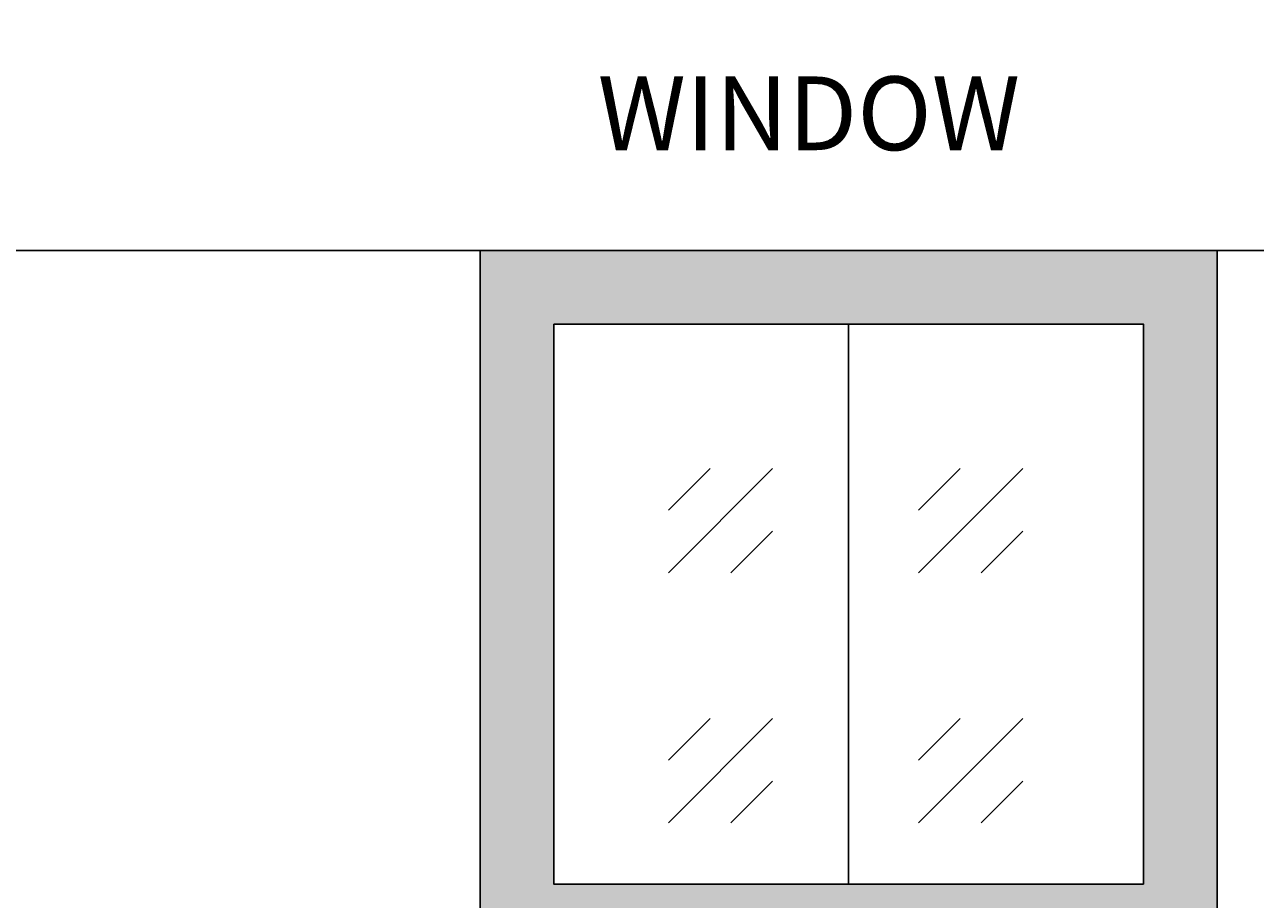
# Model space of a CAD drawing. Units: inches. Extents: x -301 to 715, y -607 to 364.
# Tile 26 of 141: x 18 to 101, y -430 to -370. Entities that reach past the tile are written whole.
import ezdxf

# ---------------------------------------------------------------- set-up
doc = ezdxf.new("R2010")
doc.units = ezdxf.units.IN
doc.header["$MEASUREMENT"] = 0
for name, color, linetype, lineweight in [('A-ANNO-DIMS', 2, 'Continuous', 18), ('A-ANNO-TEXT', 4, 'Continuous', 18), ('A-GLAZ', 2, 'Continuous', 25), ('A-SECT-PATT', 8, 'Continuous', 13)]:
    doc.layers.add(name, color=color, linetype=linetype, lineweight=lineweight)
doc.styles.get("Standard").update_dxf_attribs({"font": 'arial.ttf'})
doc.dimstyles.get("Standard").update_dxf_attribs({"dimtxt": 0.18, "dimasz": 0.18, "dimexe": 0.18, "dimexo": 0.0625, "dimgap": 0.09, "dimtad": 0, "dimtih": 1, "dimtoh": 1, "dimdec": 1, "dimzin": 0, "dimdsep": 46, "dimlunit": 4, "dimtxsty": 'Standard', "dimcen": 0.09, "dimclrd": 3, "dimclre": 4, "dimclrt": 6, "dimadec": 0, "dimazin": 0, "dimtfac": 1, "dimtdec": 1, "dimtofl": 0, "dimtmove": 0, "dimatfit": 3, "dimfxl": 1, "dimtfill": 2, "dimtfillclr": 51, "dimtolj": 1, "dimtzin": 0, "dimarcsym": 0})

# ---------------------------------------------------------------- blocks, each defined once
blk = doc.blocks.new('*D176')
at = {"layer": 'A-ANNO-DIMS', "color": 4, "lineweight": -2, "transparency": 16777216}
for p, q in [((148.28, -324.477), (215.605, -324.477)), ((-15.22, -540.477), (215.605, -540.477))]:
    blk.add_line(p, q, dxfattribs=at)
at = {"layer": 'A-ANNO-DIMS', "color": 3, "lineweight": -2, "transparency": 16777216}
for p, q in [((215.425, -324.657), (215.425, -432.296)), ((215.425, -540.297), (215.425, -432.659))]:
    blk.add_line(p, q, dxfattribs=at)
at = {"layer": 'A-ANNO-DIMS', "color": 3, "transparency": 16777216}
for points in [[(215.395, -324.657), (215.455, -324.657), (215.425, -324.477)], [(215.395, -540.297), (215.455, -540.297), (215.425, -540.477)]]:
    blk.add_solid(points, dxfattribs=at)
at = {"layer": 'Defpoints', "color": 0, "transparency": 16777216}
for p in [(148.218, -324.477), (-15.282, -540.477), (215.425, -540.477)]:
    blk.add_point(p, dxfattribs=at)
at = {"layer": 'A-ANNO-DIMS', "color": 6, "transparency": 16777216, "insert": (215.425, -432.477), "char_height": 0.18, "attachment_point": 5, "bg_fill": 1, "box_fill_scale": 1.25, "bg_fill_color": 51, "bg_fill_transparency": 0}
blk.add_mtext('\\A1;18\'-0"', dxfattribs=at)
blk = doc.blocks.new('*D187')
at = {"layer": 'A-ANNO-DIMS', "color": 4, "lineweight": -2, "transparency": 16777216}
for p, q in [((139.674, -385.477), (-266.112, -385.477)), ((143.155, -439.477), (-266.112, -439.477))]:
    blk.add_line(p, q, dxfattribs=at)
at = {"layer": 'A-ANNO-DIMS', "color": 3, "lineweight": -2, "transparency": 16777216}
for p, q in [((-265.932, -385.657), (-265.932, -412.296)), ((-265.932, -439.297), (-265.932, -412.659))]:
    blk.add_line(p, q, dxfattribs=at)
at = {"layer": 'A-ANNO-DIMS', "color": 3, "transparency": 16777216}
for points in [[(-265.962, -385.657), (-265.902, -385.657), (-265.932, -385.477)], [(-265.962, -439.297), (-265.902, -439.297), (-265.932, -439.477)]]:
    blk.add_solid(points, dxfattribs=at)
at = {"layer": 'Defpoints', "color": 0, "transparency": 16777216}
for p in [(-265.932, -385.477), (139.737, -385.477), (143.218, -439.477)]:
    blk.add_point(p, dxfattribs=at)
at = {"layer": 'A-ANNO-DIMS', "color": 6, "transparency": 16777216, "insert": (-265.932, -412.477), "char_height": 0.18, "attachment_point": 5, "bg_fill": 1, "box_fill_scale": 1.25, "bg_fill_color": 51, "bg_fill_transparency": 0}
blk.add_mtext('\\A1;4\'-6"', dxfattribs=at)

msp = doc.modelspace()

# ---------------------------------------------------------------- hatches: boundary and pattern name
at = {"layer": 'A-SECT-PATT'}
h = msp.add_hatch(color=256, dxfattribs=at)
h.dxf.hatch_style = 1
h.paths.add_polyline_path([(-138.282, -385.477), (-138.282, -433.477), (-87.981, -433.477), (-87.981, -385.477)])
h.paths.add_polyline_path([(-92.981, -390.477), (-92.981, -428.477), (-133.282, -428.477), (-133.282, -390.477)], flags=16)
h.paths.add_polyline_path([(-35.282, -385.477), (-35.282, -463.477), (12.718, -463.477), (12.718, -385.477)])
h.paths.add_polyline_path([(-30.282, -390.477), (7.718, -390.477), (7.718, -458.477), (-30.282, -458.477)], flags=16)
h.paths.add_polyline_path([(48.468, -385.477), (48.468, -433.477), (98.468, -433.477), (98.468, -385.477)])
h.paths.add_polyline_path([(93.468, -390.477), (93.468, -428.477), (53.468, -428.477), (53.468, -390.477)], flags=16)
h = msp.add_hatch(dxfattribs=at)
h.set_pattern_fill('GOST_GLASS', color=256, scale=2)
h.set_pattern_definition([(45, (10.321, 33.876), (16.97056, -2e-15), [10, -14]), (45, (14.564, 33.876), (16.97056, -2e-15), [4, -20]), (45, (10.321, 38.119), (16.97056, -2e-15), [4, -20])])
h.paths.add_polyline_path([(-113.131, -390.477), (-133.282, -390.477), (-133.282, -428.477), (-113.131, -428.477)])
h.paths.add_polyline_path([(-92.981, -390.477), (-113.131, -390.477), (-113.131, -428.477), (-92.981, -428.477)])
h.paths.add_polyline_path([(73.468, -390.477), (53.468, -390.477), (53.468, -428.477), (73.468, -428.477)])
h.paths.add_polyline_path([(93.468, -390.477), (73.468, -390.477), (73.468, -428.477), (93.468, -428.477)])

# ---------------------------------------------------------------- linework, layer by layer
at = {"layer": 'A-GLAZ'}
msp.add_line((73.468, -428.477), (73.468, -390.477), dxfattribs=at)
for points in [[(48.468, -385.477), (98.468, -385.477), (98.468, -433.477), (48.468, -433.477)], [(53.468, -390.477), (93.468, -390.477), (93.468, -428.477), (53.468, -428.477)]]:
    msp.add_lwpolyline(points, close=True, dxfattribs=at)

# ---------------------------------------------------------------- texts
at = {"layer": 'A-ANNO-TEXT', "insert": (56.443, -373.681), "char_height": 5, "attachment_point": 1}
msp.add_mtext_dynamic_manual_height_columns('WINDOW', width=73.06001, gutter_width=1, heights=[0], dxfattribs=at)

# ---------------------------------------------------------------- dimensions: what is measured, and where the dimension line sits
at = {"layer": 'A-ANNO-DIMS'}
for base, p1, p2, picture, middle in [((215.425, -540.477), (148.218, -324.477), (-15.282, -540.477), '*D176', (215.425, -432.477)), ((-265.932, -385.477), (143.218, -439.477), (139.737, -385.477), '*D187', (-265.932, -412.477))]:
    dim = msp.add_linear_dim(base=base, p1=p1, p2=p2, angle=90, dimstyle='Standard', override={"dimdec": 1, "dimlfac": 1, "dimrnd": 0, "dimzin": 1, "dimdsep": 46, "dimlunit": 4, "dimfrac": 2}, dxfattribs=at)
    dim.commit()
    dim.dimension.update_dxf_attribs({"geometry": picture, "text_midpoint": middle})

doc.saveas('drawing.dxf')
